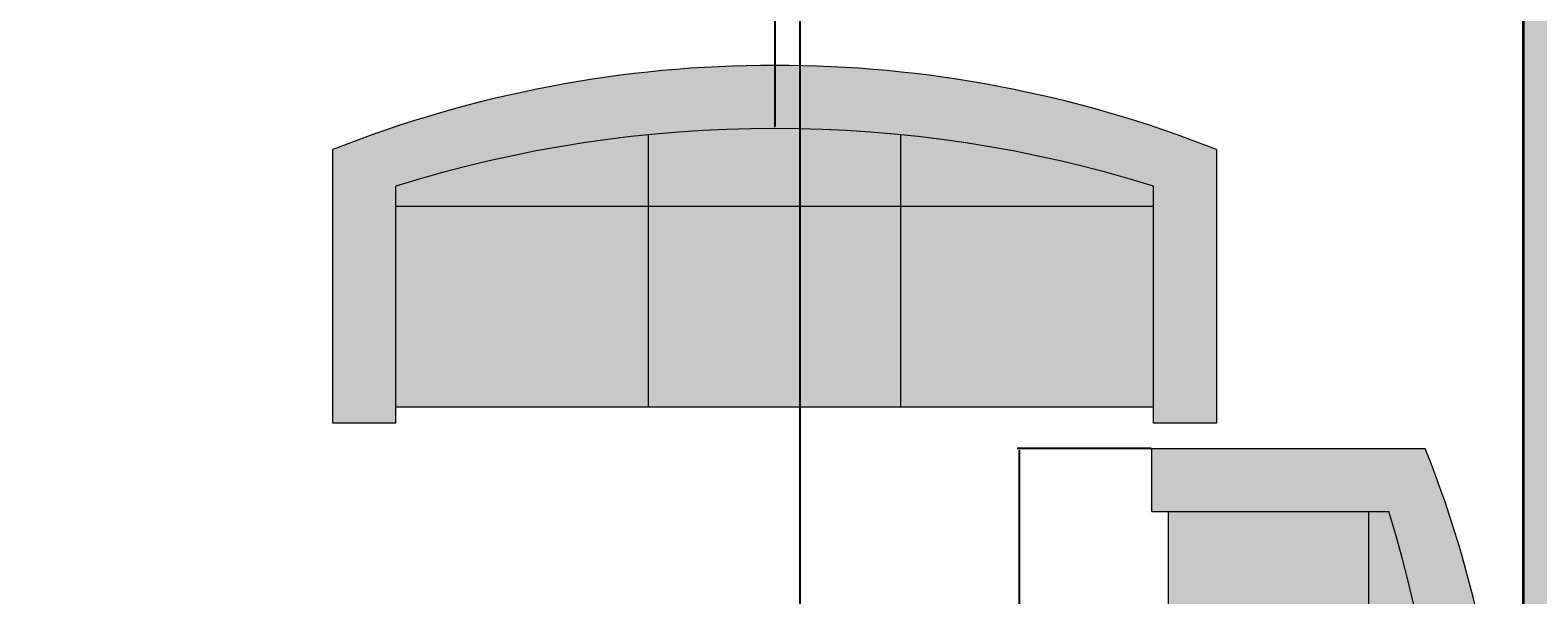
# Model space of a CAD drawing. Units: inches. Extents: x 2549 to 3108, y 1683 to 2362.
# Tile 28 of 30: x 2893 to 3036, y 2080 to 2134. Entities that reach past the tile are written whole.
import ezdxf

# ---------------------------------------------------------------- set-up
doc = ezdxf.new("R2010")
doc.units = ezdxf.units.IN
for name, color, linetype, lineweight in [('A-ANNO-DIMS', 2, 'Continuous', 18), ('A-FURN', 8, 'Continuous', 18), ('A-FURN-PATT', 9, 'Continuous', 13), ('A-WALL', 7, 'Continuous', 35), ('A-WALL-PATT', 89, 'Continuous', 13)]:
    doc.layers.add(name, color=color, linetype=linetype, lineweight=lineweight)
doc.layers.add('C-PKNG-VEHI-PATT', color=251, linetype='Continuous', lineweight=13, true_color=0x636466)
doc.layers.add('C-PVMT-PATT', color=9, linetype='Continuous', lineweight=13, true_color=0xc7c8ca)
doc.styles.get("Standard").update_dxf_attribs({"font": 'arial.ttf'})
doc.dimstyles.get("Standard").update_dxf_attribs({"dimtxt": 0.18, "dimasz": 0.18, "dimexe": 0.18, "dimexo": 0.0625, "dimgap": 0.09, "dimtad": 0, "dimtih": 1, "dimtoh": 1, "dimdec": 4, "dimzin": 0, "dimdsep": 46, "dimtxsty": 'Standard', "dimcen": 0.09, "dimadec": 0, "dimazin": 0, "dimtfac": 1, "dimtdec": 4, "dimtofl": 0, "dimtmove": 0, "dimatfit": 3, "dimfxl": 1, "dimtolj": 1, "dimtzin": 0, "dimarcsym": 0})

# ---------------------------------------------------------------- blocks, each defined once
blk = doc.blocks.new('Sofa - Roundback 7 ft.')
for p, q in [((-12.00002, -32.4421), (-12.00003, -6.5971)), ((11.99997, -32.4421), (11.99998, -6.5971)), ((-36.000027, -34), (-36.000027, -11.4696)), ((35.99998, -34), (35.99998, -11.4696)), ((-35.999844, -13.3819), (35.9998, -13.3819)), ((-36.000027, -32.4421), (35.99998, -32.4421))]:
    blk.add_line(p, q)
for points in [[(-36.000027, -34), (-42.000027, -34), (-42.000027, -8)], [(41.99998, -8), (41.99998, -34), (35.99998, -34)]]:
    blk.add_lwpolyline(points)
for centre, radius, start, end in [((0, -114.25), 114.25, 68.43141, 111.5686), ((-0.00001, -127.1968), 121.1968, 72.72033, 107.2797)]:
    blk.add_arc(centre, radius, start, end)
blk = doc.blocks.new('*D16')
at = {"layer": 'A-ANNO-DIMS', "color": 0, "lineweight": -2, "transparency": 16777216}
for p, q in [((2999.28, 2094.09), (2986.57, 2094.09)), ((2986.75, 2093.91), (2986.75, 2052.27)), ((2986.75, 2010.27), (2986.75, 2051.91)), ((2999.28, 2010.09), (2986.57, 2010.09))]:
    blk.add_line(p, q, dxfattribs=at)
at = {"layer": 'A-ANNO-DIMS', "color": 0, "transparency": 16777216}
for points in [[(2986.72, 2093.91), (2986.78, 2093.91), (2986.75, 2094.09)], [(2986.72, 2010.27), (2986.78, 2010.27), (2986.75, 2010.09)]]:
    blk.add_solid(points, dxfattribs=at)
at = {"layer": 'Defpoints', "color": 0, "transparency": 16777216}
for p in [(2999.35, 2094.09), (2986.75, 2010.09), (2999.35, 2010.09)]:
    blk.add_point(p, dxfattribs=at)
at = {"layer": 'A-ANNO-DIMS', "color": 0, "transparency": 16777216, "insert": (2986.75, 2052.09), "char_height": 0.18, "attachment_point": 5}
blk.add_mtext('\\A1;SOFA 84 TYP.', dxfattribs=at)
blk = doc.blocks.new('*D46')
at = {"layer": 'A-ANNO-DIMS', "color": 0, "lineweight": -2, "transparency": 16777216}
for p, q in [((2812.64, 2140.46), (2812.64, 1683.44)), ((3034.64, 2134.46), (3034.64, 1683.44)), ((2812.82, 1683.62), (2923.35, 1683.62)), ((3034.46, 1683.62), (2923.93, 1683.62))]:
    blk.add_line(p, q, dxfattribs=at)
at = {"layer": 'A-ANNO-DIMS', "color": 0, "transparency": 16777216}
for points in [[(2812.82, 1683.65), (2812.82, 1683.59), (2812.64, 1683.62)], [(3034.46, 1683.65), (3034.46, 1683.59), (3034.64, 1683.62)]]:
    blk.add_solid(points, dxfattribs=at)
at = {"layer": 'Defpoints', "color": 0, "transparency": 16777216}
for p in [(2812.64, 2140.52), (3034.64, 2134.52), (3034.64, 1683.62)]:
    blk.add_point(p, dxfattribs=at)
at = {"layer": 'A-ANNO-DIMS', "color": 0, "transparency": 16777216, "insert": (2923.64, 1683.62), "char_height": 0.18, "attachment_point": 5}
blk.add_mtext('\\A1;222', dxfattribs=at)
blk = doc.blocks.new('*D57')
at = {"layer": 'A-ANNO-DIMS', "color": 0, "lineweight": -2, "transparency": 16777216}
for p, q in [((2965.94, 1936.59), (2965.94, 2362.32)), ((2966.12, 2362.14), (2999.91, 2362.14)), ((3034.46, 2362.14), (3000.67, 2362.14)), ((3034.64, 1936.59), (3034.64, 2362.32))]:
    blk.add_line(p, q, dxfattribs=at)
at = {"layer": 'A-ANNO-DIMS', "color": 0, "transparency": 16777216}
for points in [[(2966.12, 2362.17), (2966.12, 2362.11), (2965.94, 2362.14)], [(3034.46, 2362.17), (3034.46, 2362.11), (3034.64, 2362.14)]]:
    blk.add_solid(points, dxfattribs=at)
at = {"layer": 'Defpoints', "color": 0, "transparency": 16777216}
for p in [(3034.64, 2362.14), (2965.94, 1936.52), (3034.64, 1936.52)]:
    blk.add_point(p, dxfattribs=at)
at = {"layer": 'A-ANNO-DIMS', "color": 0, "transparency": 16777216, "insert": (3000.29, 2362.14), "char_height": 0.18, "attachment_point": 5}
blk.add_mtext('\\A1;68.71', dxfattribs=at)
blk = doc.blocks.new('*D63')
at = {"layer": 'A-ANNO-DIMS', "color": 0, "lineweight": -2, "transparency": 16777216}
for p, q in [((2963.33, 2197.21), (2963.51, 2197.21)), ((2963.51, 2197.21), (2963.51, 2124.68)), ((2963.51, 2003.21), (2963.51, 2003.39)), ((2963.42, 2003.3), (2963.6, 2003.3))]:
    blk.add_line(p, q, dxfattribs=at)
at = {"layer": 'A-ANNO-DIMS', "color": 0, "transparency": 16777216}
blk.add_solid([(2963.54, 2124.68), (2963.48, 2124.68), (2963.51, 2124.5)], dxfattribs=at)
at = {"layer": 'Defpoints', "color": 0, "transparency": 16777216}
for p in [(2963.51, 2124.5), (2963.51, 2003.3)]:
    blk.add_point(p, dxfattribs=at)
at = {"layer": 'A-ANNO-DIMS', "color": 0, "transparency": 16777216, "insert": (2962.65, 2197.21), "char_height": 0.18, "attachment_point": 5}
blk.add_mtext('\\A1;2X R121.2', dxfattribs=at)

msp = doc.modelspace()

# ---------------------------------------------------------------- hatches: boundary and pattern name
at = {"layer": 'A-FURN-PATT', "transparency": 33554684}
h = msp.add_hatch(color=256, dxfattribs=at)
h.dxf.hatch_style = 1
h.paths.add_polyline_path([(2927.5085, 2119.0252, -0.15194781), (2999.5085, 2119.0252), (2999.5085, 2096.4953), (3005.5085, 2096.4953), (3005.5085, 2122.4953, 0.19047621), (2921.5085, 2122.4953), (2921.5085, 2096.4953), (2927.5085, 2096.4953)])
h.paths.add_polyline_path([(2951.5085, 2117.1134), (2927.5085, 2117.1134), (2927.5085, 2098.0532), (2951.5085, 2098.0532)], flags=17)
h.paths.add_polyline_path([(2975.5085, 2117.1134), (2951.5085, 2117.1134), (2951.5085, 2098.0532), (2975.5085, 2098.0532)], flags=17)
h.paths.add_polyline_path([(2975.5085, 2123.8998, 0.04962821), (2951.5085, 2123.8998), (2951.5085, 2117.1134), (2975.5085, 2117.1134)], flags=17)
h.paths.add_polyline_path([(2951.5085, 2123.8998, 0.05064665), (2927.5085, 2119.0252), (2927.5085, 2117.1134), (2951.5085, 2117.1134)], flags=17)
h.paths.add_polyline_path([(2975.5085, 2123.8998), (2975.5085, 2117.1134), (2999.5085, 2117.1134), (2999.5085, 2119.0252, 0.05064665)], flags=17)
h.paths.add_polyline_path([(2999.5085, 2117.1134), (2975.5085, 2117.1134), (2975.5085, 2098.0532), (2999.5085, 2098.0532)], flags=17)
h.paths.add_polyline_path([(3019.9651, 2088.0905), (3000.9049, 2088.0905), (3000.9049, 2064.0905), (3019.9651, 2064.0905)], flags=17)
h.paths.add_polyline_path([(3025.347, 2094.0905), (2999.347, 2094.0905), (2999.347, 2088.0905), (3021.8769, 2088.0905, -0.15194781), (3021.8769, 2016.0905), (2999.347, 2016.0905), (2999.347, 2010.0905), (3025.347, 2010.0905, 0.19047621)])
h.paths.add_polyline_path([(3021.8769, 2088.0905), (3019.9651, 2088.0905), (3019.9651, 2064.0905), (3026.7514, 2064.0905, 0.05064665)], flags=17)
h.paths.add_polyline_path([(3026.7514, 2064.0905), (3019.9651, 2064.0905), (3019.9651, 2040.0905), (3026.7514, 2040.0905, 0.04962821)], flags=17)
h.paths.add_polyline_path([(3019.9651, 2064.0905), (3000.9049, 2064.0905), (3000.9049, 2040.0905), (3019.9651, 2040.0905)], flags=17)
h.paths.add_polyline_path([(3019.9651, 2040.0905), (3000.9049, 2040.0905), (3000.9049, 2016.0905), (3019.9651, 2016.0905)], flags=17)
h.paths.add_polyline_path([(3026.7514, 2040.0905), (3019.9651, 2040.0905), (3019.9651, 2016.0905), (3021.8769, 2016.0905, 0.05064665)], flags=17)
at = {"layer": 'A-WALL-PATT'}
h = msp.add_hatch(color=256, dxfattribs=at)
h.dxf.hatch_style = 1
h.paths.add_polyline_path([(2638.6427, 2272.5237), (3034.6427, 2272.5237), (3034.6427, 1936.5237), (3043.6427, 1936.5237), (3043.6427, 2281.5237), (2629.6427, 2281.5237), (2629.6427, 2074.5237), (2812.6427, 2074.5237), (2812.6427, 2140.5237), (2785.7177, 2140.5237), (2785.7177, 2134.5237), (2806.6427, 2134.5237), (2806.6427, 2080.5237), (2638.6427, 2080.5237)])
h.paths.add_polyline_path([(2638.6427, 1972.5237), (2662.6427, 1972.5237), (2662.6427, 2041.0557), (2653.6427, 2041.0557), (2653.6427, 1978.5237), (2629.6427, 1978.5237), (2629.6427, 1795.5237), (2662.6427, 1795.5237), (2881.6427, 1795.5237), (2881.6427, 1936.5237), (2965.9351, 1936.5237), (2965.9351, 1974.5439), (2959.9351, 1974.5439), (2959.9351, 1945.5237), (2881.6427, 1945.5237), (2872.6427, 1945.5237), (2872.6427, 1804.5237), (2662.6427, 1804.5237), (2638.6427, 1804.5237)])
at = {"layer": 'C-PKNG-VEHI-PATT'}
h = msp.add_hatch(color=256, dxfattribs=at)
h.dxf.hatch_style = 1
edge = h.paths.add_edge_path()
edge.add_ellipse((2935.7258, 1791.964), major_axis=(-50.66, 0), ratio=0.84230387, start_angle=248.165046, end_angle=265.722579)
edge.add_line((2938.911, 1834.5507), (2925.8653, 1834.5507))
edge.add_ellipse((2929.0505, 1791.964), major_axis=(50.66, 0), ratio=0.84230387, start_angle=94.277421, end_angle=111.834954)
edge.add_line((2912.8508, 1832.3947), (2914.2044, 1822.2495))
edge.add_ellipse((2930.6538, 1783.1023), major_axis=(-49.3014, 0), ratio=0.84230387, start_angle=-85.12993, end_angle=-67.208085, ccw=False)
edge.add_line((2927.1247, 1824.5225), (2937.6516, 1824.5225))
edge.add_ellipse((2934.1225, 1783.1023), major_axis=(49.3014, 0), ratio=0.84230387, start_angle=67.208085, end_angle=85.12993, ccw=False)
edge.add_line((2950.5719, 1822.2495), (2951.9255, 1832.3947))
edge = h.paths.add_edge_path()
edge.add_ellipse((2903.4793, 1857.3351), major_axis=(-34.7979, 0), ratio=0.84230387, start_angle=180, end_angle=209.43857)
edge.add_ellipse((2961.297, 1857.3351), major_axis=(34.7979, 0), ratio=0.84230387, start_angle=150.56143, end_angle=180)
edge.add_line((2926.4991, 1857.3351), (2926.4991, 1843.7609))
edge.add_ellipse((2924.1251, 1844.3143), major_axis=(-0.2209, 3.9278), ratio=0.60383358, start_angle=89.002014, end_angle=253.657408, ccw=False)
edge.add_line((2921.7512, 1844.2222), (2921.7512, 1853.3975))
edge.add_line((2921.7512, 1853.3975), (2925.269, 1855.8484))
edge.add_ellipse((2925.4782, 1855.4931), major_axis=(0.4584, 0), ratio=0.84230387, start_angle=90, end_angle=134.480211, ccw=False)
edge.add_line((2925.4782, 1855.8792), (2926.4991, 1855.8792))
edge.add_line((2926.4991, 1855.8792), (2926.4991, 1857.3351))
edge.add_ellipse((2961.297, 1857.3351), major_axis=(34.7979, 0), ratio=0.84230387, start_angle=150.56143, end_angle=180, ccw=False)
edge.add_line((2932.3882, 1873.6501), (2932.3882, 1875.7801))
edge.add_ellipse((2932.3882, 1875.3939), major_axis=(0.4584, 0), ratio=0.84230387, start_angle=90, end_angle=127.93313)
edge.add_line((2932.1366, 1875.7167), (2928.5915, 1873.7564))
edge.add_ellipse((2899.9271, 2002.4692), major_axis=(155.4756, 0), ratio=0.84230387, start_angle=-80.743434, end_angle=-77.445067, ccw=False)
edge.add_ellipse((2949.4402, 1715.2151), major_axis=(-189.1422, 0), ratio=0.84230387, start_angle=-79.790461, end_angle=-77.555373)
edge.add_ellipse((3300.3614, 1852.5642), major_axis=(-386.1662, 0), ratio=0.84230387, start_angle=-2.863715, end_angle=2.198541)
edge.add_ellipse((2929.0505, 1792.5159), major_axis=(-55.6192, 0), ratio=0.84230387, start_angle=-85.917589, end_angle=-72.280047, ccw=False)
edge.add_line((2925.7129, 1839.2798), (2939.0634, 1839.2798))
edge.add_ellipse((2935.7258, 1792.5159), major_axis=(55.6192, 0), ratio=0.84230387, start_angle=72.280047, end_angle=85.917589, ccw=False)
edge.add_ellipse((2564.4149, 1852.5642), major_axis=(-386.1662, 0), ratio=0.84230387, start_angle=177.801459, end_angle=182.863715)
edge.add_ellipse((2915.3361, 1715.2151), major_axis=(189.1422, 0), ratio=0.84230387, start_angle=77.555373, end_angle=79.790461)
edge.add_ellipse((2964.8492, 2002.4692), major_axis=(-155.4756, 0), ratio=0.84230387, start_angle=77.445067, end_angle=80.743434, ccw=False)
edge.add_line((2936.1848, 1873.7564), (2932.6397, 1875.7167))
edge.add_ellipse((2932.3882, 1875.3939), major_axis=(0.4584, 0), ratio=0.84230387, start_angle=52.06687, end_angle=90)
edge.add_line((2932.3882, 1875.7801), (2932.3882, 1873.6501))
edge.add_ellipse((2903.4793, 1857.3351), major_axis=(-34.7979, 0), ratio=0.84230387, start_angle=180, end_angle=209.43857, ccw=False)
edge.add_line((2938.2772, 1857.3351), (2938.2772, 1855.8792))
edge.add_line((2938.2772, 1855.8792), (2939.4059, 1855.8792))
edge.add_ellipse((2939.2981, 1855.4931), major_axis=(-0.4584, 0), ratio=0.84230387, start_angle=225.519789, end_angle=270, ccw=False)
edge.add_line((2939.5903, 1855.7906), (2943.0251, 1853.3975))
edge.add_line((2943.0251, 1853.3975), (2943.0251, 1844.2222))
edge.add_ellipse((2940.6512, 1844.3143), major_axis=(0.2209, 3.9278), ratio=0.60383358, start_angle=106.342592, end_angle=270.997986, ccw=False)
edge.add_line((2938.2772, 1843.7609), (2938.2772, 1857.3351))
edge = h.paths.add_edge_path()
edge.add_ellipse((2932.3882, 1865.1973), major_axis=(91.081, 0), ratio=0.84230387, start_angle=256.401865, end_angle=283.598135, ccw=False)
edge.add_line((2914.2044, 1790.0239), (2914.2044, 1778.3622))
edge.add_ellipse((2932.3882, 1853.5356), major_axis=(91.081, 0), ratio=0.84230387, start_angle=256.401865, end_angle=283.598135)
edge.add_line((2950.5719, 1778.3622), (2950.5719, 1790.0239))
edge = h.paths.add_edge_path()
edge.add_ellipse((2948.7383, 1772.3145), major_axis=(1.8336, 0), ratio=0.84230387, start_angle=0, end_angle=90)
edge.add_line((2948.7383, 1773.859), (2916.038, 1773.859))
edge.add_ellipse((2916.038, 1772.3145), major_axis=(1.8336, 0), ratio=0.84230387, start_angle=90, end_angle=180)
edge.add_line((2914.2044, 1772.3145), (2914.2044, 1760.2558))
edge.add_line((2914.2044, 1760.2558), (2950.5719, 1760.2558))
edge.add_line((2950.5719, 1760.2558), (2950.5719, 1772.3145))
h.paths.add_polyline_path([(2748.8496, 2101.6383), (2798.148, 2101.6383), (2798.148, 2111.4248), (2748.8496, 2111.4248)], flags=9)
h.paths.add_polyline_path([(2685.2081, 2101.489), (2719.3253, 2101.489), (2719.3253, 2111.2819), (2685.2081, 2111.2819)], flags=9)
h.paths.add_polyline_path([(2814.6852, 1907.1328), (2847.8384, 1907.1328), (2847.8384, 1916.9258), (2814.6852, 1916.9258)], flags=9)
h.paths.add_polyline_path([(2814.3906, 1835.5864), (2848.0172, 1835.5864), (2848.0172, 1845.3794), (2814.3906, 1845.3794)], flags=9)
h.paths.add_polyline_path([(2800.5245, 1759.1674), (2853.7435, 1759.1674), (2853.7435, 1768.954), (2800.5245, 1768.954)], flags=9)
h.paths.add_polyline_path([(2972.4611, 1807.3305), (3015.3943, 1807.3305), (3015.3943, 1817.117), (2972.4611, 1817.117)], flags=9)
h.paths.add_polyline_path([(2902.3327, 1888.6731), (2937.9131, 1888.6731), (2937.9131, 1898.4661), (2902.3327, 1898.4661)], flags=9)
h.paths.add_polyline_path([(2712.1779, 1878.9039), (2754.1257, 1878.9039), (2754.1257, 1888.6904), (2712.1779, 1888.6904)], flags=9)
h.paths.add_polyline_path([(2614.0056, 2012.812), (2650.0251, 2012.812), (2650.0251, 2022.4371), (2614.0056, 2022.4371)], flags=9)
h.paths.add_polyline_path([(2713.3129, 2003.1645), (2747.4237, 2003.1645), (2747.4237, 2012.951), (2713.3129, 2012.951)], flags=9)
h.paths.add_polyline_path([(2950.1379, 2001.6934), (2982.2992, 2001.6934), (2982.2992, 2011.48), (2950.1379, 2011.48)], flags=9)
h.paths.add_polyline_path([(2940.864, 2238.5537), (2997.5066, 2238.5537), (2997.5066, 2248.3466), (2940.864, 2248.3466)], flags=9)
h.paths.add_polyline_path([(2821.5457, 2202.8348), (2855.663, 2202.8348), (2855.663, 2212.6278), (2821.5457, 2212.6278)], flags=9)
h.paths.add_polyline_path([(2661.8026, 2238.6249), (2718.4451, 2238.6249), (2718.4451, 2248.4179), (2661.8026, 2248.4179)], flags=9)
at = {"layer": 'C-PVMT-PATT'}
h = msp.add_hatch(color=256, dxfattribs=at)
h.dxf.hatch_style = 1
h.paths.add_polyline_path([(3067.6427, 2305.5237), (2605.6427, 2305.5237), (2605.6427, 2074.5237), (2629.6427, 2074.5237), (2629.6427, 2281.5237), (3043.6427, 2281.5237), (3043.6427, 1885.5237), (3043.6427, 1872.8745), (3031.1672, 1872.8745), (3031.1672, 1862.5731), (2995.8054, 1862.5731), (2995.8054, 1872.8745), (2983.1752, 1872.8745), (2983.1752, 1885.5237), (2881.6427, 1885.5237), (2881.6427, 1795.5237), (2751.0977, 1795.5237), (2751.0977, 1761.5237), (2786.1577, 1761.5237), (2786.1577, 1723.5237), (2881.84, 1723.5237), (2881.84, 1714.5237), (3067.6427, 1714.5237), (3067.6427, 1723.5237)])
edge = h.paths.add_edge_path(flags=16)
edge.add_ellipse((2949.4402, 1710.9683), major_axis=(-194.1014, 0), ratio=0.84230387, start_angle=-77.874034, end_angle=-76.219471, ccw=False)
edge.add_ellipse((2949.4402, 1715.2151), major_axis=(-189.1422, 0), ratio=0.84230387, start_angle=-79.790461, end_angle=-77.555373, ccw=False)
edge.add_ellipse((2899.9271, 2002.4692), major_axis=(155.4756, 0), ratio=0.84230387, start_angle=-80.743434, end_angle=-77.445067)
edge.add_line((2928.5915, 1873.7564), (2932.3882, 1875.8558))
edge.add_line((2932.3882, 1875.8558), (2936.1848, 1873.7564))
edge.add_ellipse((2964.8492, 2002.4692), major_axis=(-155.4756, 0), ratio=0.84230387, start_angle=77.445067, end_angle=80.743434)
edge.add_ellipse((2915.3361, 1715.2151), major_axis=(189.1422, 0), ratio=0.84230387, start_angle=77.555373, end_angle=79.790461, ccw=False)
edge.add_ellipse((2915.3361, 1710.9683), major_axis=(-194.1014, 0), ratio=0.84230387, start_angle=256.219471, end_angle=257.874034, ccw=False)
edge.add_ellipse((2628.2871, 1850.2612), major_axis=(-327.2532, 0), ratio=0.84230387, start_angle=182.17995, end_angle=183.650428, ccw=False)
edge.add_ellipse((2955.5637, 1861.9334), major_axis=(-0.9168, 0), ratio=0.84230387, start_angle=180, end_angle=270, ccw=False)
edge.add_line((2956.4805, 1862.3857), (2956.4805, 1846.4866))
edge.add_ellipse((2955.5637, 1846.939), major_axis=(-0.9168, 0), ratio=0.84230387, start_angle=90, end_angle=180, ccw=False)
edge.add_ellipse((-3607.0606, 1835.832), major_axis=(-6562.6242, 0), ratio=0.84230387, start_angle=179.61613322, end_angle=180.09022909, ccw=False)
edge.add_ellipse((2955.5637, 1791.0926), major_axis=(0.9168, 0), ratio=0.84230387, start_angle=0, end_angle=90, ccw=False)
edge.add_line((2956.4805, 1791.545), (2956.4805, 1775.6459))
edge.add_ellipse((2955.5637, 1776.0982), major_axis=(0.9168, 0), ratio=0.84230387, start_angle=270, end_angle=360, ccw=False)
edge.add_ellipse((-3607.0606, 1835.832), major_axis=(-6562.6242, 0), ratio=0.84230387, start_angle=179.3813568, end_angle=179.47172853, ccw=False)
edge.add_ellipse((2954.5907, 1763.8768), major_axis=(-1.3752, 0), ratio=0.84230387, start_angle=179.371763, end_angle=248.464757, ccw=False)
edge.add_ellipse((-3607.519, 1835.832), major_axis=(-6564.0409, 0), ratio=0.842303863, start_angle=179.35344594, end_angle=179.37176282, ccw=False)
edge.add_ellipse((2952.6829, 1761.8002), major_axis=(3.2503, 0), ratio=0.84230387, start_angle=-90, end_angle=-0.646554, ccw=False)
edge.add_line((2952.6829, 1759.0625), (2912.0934, 1759.0625))
edge.add_ellipse((2912.0934, 1761.8002), major_axis=(3.2503, 0), ratio=0.84230387, start_angle=180.646554, end_angle=270, ccw=False)
edge.add_ellipse((9472.2953, 1835.832), major_axis=(-6564.0409, 0), ratio=0.842303871, start_angle=0.62823722, end_angle=0.6465541, ccw=False)
edge.add_ellipse((2910.1856, 1763.8768), major_axis=(1.3752, 0), ratio=0.84230387, start_angle=111.535244, end_angle=180.628237, ccw=False)
edge.add_ellipse((9471.8369, 1835.832), major_axis=(-6562.6242, 0), ratio=0.84230387, start_angle=0.52827147, end_angle=0.6465541, ccw=False)
edge.add_ellipse((2909.2126, 1776.0982), major_axis=(-0.9168, 0), ratio=0.84230387, start_angle=0, end_angle=90, ccw=False)
edge.add_line((2908.2958, 1775.6459), (2908.2958, 1791.545))
edge.add_ellipse((2909.2126, 1791.0926), major_axis=(-0.9168, 0), ratio=0.84230387, start_angle=-90, end_angle=0, ccw=False)
edge.add_ellipse((9471.8369, 1835.832), major_axis=(-6562.6242, 0), ratio=0.84230387, start_angle=-0.09022909, end_angle=0.38386678, ccw=False)
edge.add_ellipse((2909.2126, 1846.939), major_axis=(-0.9168, 0), ratio=0.84230387, start_angle=0, end_angle=90, ccw=False)
edge.add_line((2908.2958, 1846.4866), (2908.2958, 1862.3857))
edge.add_ellipse((2909.2126, 1861.9334), major_axis=(0.9168, 0), ratio=0.84230387, start_angle=90, end_angle=180, ccw=False)
edge.add_ellipse((3236.4892, 1850.2612), major_axis=(327.2532, 0), ratio=0.84230387, start_angle=176.349572, end_angle=177.82005, ccw=False)
edge = h.paths.add_edge_path(flags=0)
edge.add_ellipse((2903.4793, 1857.3351), major_axis=(-34.7979, 0), ratio=0.84230387, start_angle=180, end_angle=209.43857, ccw=False)
edge.add_line((2938.2772, 1857.3351), (2938.2772, 1855.8792))
edge.add_line((2938.2772, 1855.8792), (2939.4631, 1855.8792))
edge.add_line((2939.4631, 1855.8792), (2943.0251, 1853.3975))
edge.add_line((2943.0251, 1853.3975), (2943.0251, 1844.2222))
edge.add_ellipse((2940.6512, 1844.3143), major_axis=(0.2209, 3.9278), ratio=0.60383358, start_angle=106.342592, end_angle=270.997986, ccw=False)
edge.add_line((2938.2772, 1843.7609), (2938.2772, 1857.3351))
edge.add_ellipse((2903.4793, 1857.3351), major_axis=(-34.7979, 0), ratio=0.84230387, start_angle=180, end_angle=209.43857)
edge.add_ellipse((2961.297, 1857.3351), major_axis=(34.7979, 0), ratio=0.84230387, start_angle=150.56143, end_angle=180)
edge.add_line((2926.4991, 1857.3351), (2926.4991, 1843.7609))
edge.add_ellipse((2924.1251, 1844.3143), major_axis=(-0.2209, 3.9278), ratio=0.60383358, start_angle=89.002014, end_angle=253.657408, ccw=False)
edge.add_line((2921.7512, 1844.2222), (2921.7512, 1853.3975))
edge.add_line((2921.7512, 1853.3975), (2925.3132, 1855.8792))
edge.add_line((2925.3132, 1855.8792), (2926.4991, 1855.8792))
edge.add_line((2926.4991, 1855.8792), (2926.4991, 1857.3351))
edge.add_ellipse((2961.297, 1857.3351), major_axis=(34.7979, 0), ratio=0.84230387, start_angle=150.56143, end_angle=180, ccw=False)
edge = h.paths.add_edge_path(flags=0)
edge.add_ellipse((2929.0505, 1791.964), major_axis=(50.66, 0), ratio=0.84230387, start_angle=94.277421, end_angle=111.834954, ccw=False)
edge.add_line((2925.8653, 1834.5507), (2938.911, 1834.5507))
edge.add_ellipse((2935.7258, 1791.964), major_axis=(-50.66, 0), ratio=0.84230387, start_angle=248.165046, end_angle=265.722579, ccw=False)
edge.add_line((2951.9255, 1832.3947), (2950.5719, 1822.2495))
edge.add_ellipse((2934.1225, 1783.1023), major_axis=(49.3014, 0), ratio=0.84230387, start_angle=67.208085, end_angle=85.12993)
edge.add_line((2937.6516, 1824.5225), (2927.1247, 1824.5225))
edge.add_ellipse((2930.6538, 1783.1023), major_axis=(-49.3014, 0), ratio=0.84230387, start_angle=-85.12993, end_angle=-67.208085)
edge.add_line((2914.2044, 1822.2495), (2912.8508, 1832.3947))
edge = h.paths.add_edge_path(flags=0)
edge.add_line((2910.1338, 1829.4651), (2912.6432, 1821.2711))
edge.add_ellipse((5203.7787, 1816.4367), major_axis=(-2291.1426, 0), ratio=0.84230387, start_angle=-0.1208974, end_angle=0.3640763)
edge.add_line((2912.7012, 1801.8782), (2910.3305, 1792.5698))
edge.add_ellipse((9471.8369, 1835.832), major_axis=(-6561.7074, 0), ratio=0.84230387, start_angle=0.05559431, end_angle=0.37776419, ccw=False)
edge = h.paths.add_edge_path(flags=0)
edge.add_ellipse((-3607.0606, 1835.832), major_axis=(6561.7074, 0), ratio=0.84230387, start_angle=-0.37776419, end_angle=-0.05559431, ccw=False)
edge.add_line((2954.4458, 1792.5698), (2952.0751, 1801.8782))
edge.add_ellipse((660.9976, 1816.4367), major_axis=(2291.1426, 0), ratio=0.84230387, start_angle=-0.3640763, end_angle=0.1208974)
edge.add_line((2952.1331, 1821.2711), (2954.6425, 1829.4651))
edge = h.paths.add_edge_path(flags=0)
edge.add_ellipse((2932.3882, 1865.1973), major_axis=(91.081, 0), ratio=0.84230387, start_angle=256.401865, end_angle=283.598135)
edge.add_line((2950.5719, 1790.0239), (2950.5719, 1778.3622))
edge.add_ellipse((2932.3882, 1853.5356), major_axis=(91.081, 0), ratio=0.84230387, start_angle=256.401865, end_angle=283.598135, ccw=False)
edge.add_line((2914.2044, 1778.3622), (2914.2044, 1790.0239))
edge = h.paths.add_edge_path(flags=0)
edge.add_line((2916.038, 1773.859), (2948.7383, 1773.859))
edge.add_ellipse((2948.7383, 1772.3145), major_axis=(1.8336, 0), ratio=0.84230387, start_angle=0, end_angle=90, ccw=False)
edge.add_line((2950.5719, 1772.3145), (2950.5719, 1760.2558))
edge.add_line((2950.5719, 1760.2558), (2914.2044, 1760.2558))
edge.add_line((2914.2044, 1760.2558), (2914.2044, 1772.3145))
edge.add_ellipse((2916.038, 1772.3145), major_axis=(1.8336, 0), ratio=0.84230387, start_angle=90, end_angle=180, ccw=False)
h.paths.add_polyline_path([(2629.6427, 1978.5237), (2605.6427, 1978.5237), (2605.6427, 1723.5237), (2629.6427, 1723.5237), (2629.6427, 1795.5237)], flags=17)
h.paths.add_polyline_path([(2800.5245, 1759.1674), (2853.7435, 1759.1674), (2853.7435, 1768.954), (2800.5245, 1768.954)], flags=24)
h.paths.add_polyline_path([(2972.4611, 1807.3305), (3015.3943, 1807.3305), (3015.3943, 1817.117), (2972.4611, 1817.117)], flags=24)

# ---------------------------------------------------------------- linework, layer by layer
at = {"layer": 'A-WALL'}
msp.add_line((3034.6427, 2272.5237), (3034.6427, 1936.5237), dxfattribs=at)

# ---------------------------------------------------------------- block references
at = {"layer": 'A-FURN'}
msp.add_blockref('Sofa - Roundback 7 ft.', (2963.5085, 2130.4953), dxfattribs=at)
at = {"layer": 'A-FURN', "rotation": 270}
msp.add_blockref('Sofa - Roundback 7 ft.', (3033.347, 2052.0905), dxfattribs=at)

# ---------------------------------------------------------------- dimensions: what is measured, and where the dimension line sits
at = {"layer": 'A-ANNO-DIMS'}
for base, p1, p2, override, picture, middle in [((3034.6427, 2362.1425), (2965.9351, 1936.5237), (3034.6427, 1936.5237), {"dimdec": 2, "dimlfac": 1, "dimrnd": 0, "dimzin": 0, "dimdsep": 46, "dimlunit": 2}, '*D57', (3000.2889, 2362.1425)), ((3034.6427, 1683.6237), (2812.6427, 2140.5237), (3034.6427, 2134.5237), {"dimdec": 0, "dimlfac": 1, "dimrnd": 0, "dimzin": 0, "dimdsep": 46, "dimlunit": 2}, '*D46', (2923.6427, 1683.6237))]:
    dim = msp.add_linear_dim(base=base, p1=p1, p2=p2, dimstyle='Standard', override=override, dxfattribs=at)
    dim.commit()
    dim.dimension.update_dxf_attribs({"geometry": picture, "text_midpoint": middle})
dim = msp.add_radius_dim(center=(2963.5085, 2003.2985), mpoint=(2963.508, 2124.4953), text='2X <>', dimstyle='Standard', override={"dimdec": 1, "dimlfac": 1, "dimrnd": 0, "dimzin": 0, "dimdsep": 46, "dimlunit": 2}, dxfattribs=at)
dim.commit()
dim.dimension.update_dxf_attribs({"geometry": '*D63', "text_midpoint": (2962.6539, 2197.2134), "dimtype": 164})
dim = msp.add_linear_dim(base=(2986.747, 2010.0905), p1=(2999.347, 2094.0905), p2=(2999.347, 2010.0905), angle=270, text='SOFA <> TYP.', dimstyle='Standard', override={"dimdec": 0, "dimlfac": 1, "dimrnd": 0, "dimzin": 0, "dimdsep": 46, "dimlunit": 2}, dxfattribs=at)
dim.commit()
dim.dimension.update_dxf_attribs({"geometry": '*D16', "text_midpoint": (2986.747, 2052.0905)})

doc.saveas('drawing.dxf')
